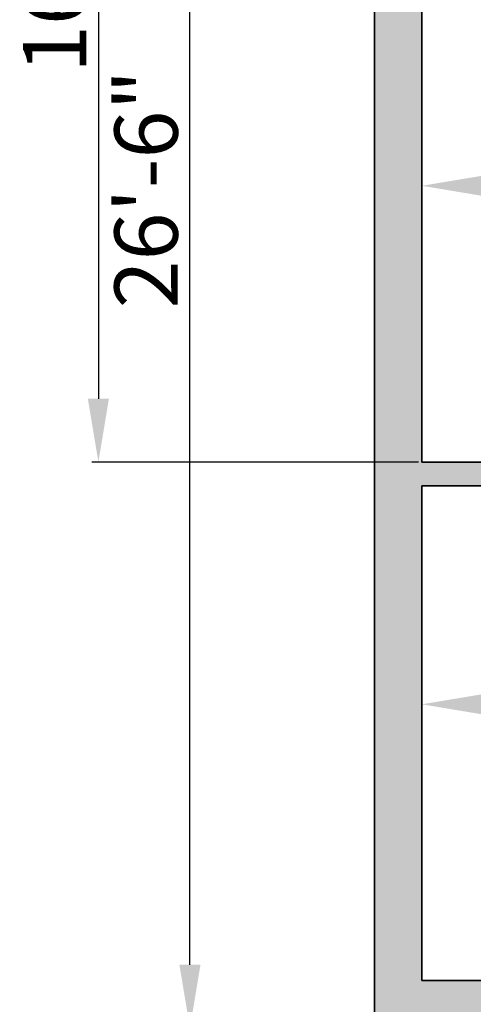
# Model space of a CAD drawing. Units: inches. Extents: x 2083 to 3317, y 1141 to 2115.
# Tile 91 of 256: x 2160 to 2246, y 1707 to 1894. Entities that reach past the tile are written whole.
import ezdxf

# ---------------------------------------------------------------- set-up
doc = ezdxf.new("R2010")
doc.units = ezdxf.units.IN
doc.layers.add('A-ANNO-DIMS', color=2, linetype='Continuous', lineweight=18)
doc.layers.add('A-WALL', color=7, linetype='Continuous', lineweight=35)
doc.layers.add('A-WALL-PATT', color=251, linetype='Continuous', lineweight=13, true_color=0x636466)
doc.styles.get("Standard").update_dxf_attribs({"font": 'arial.ttf'})
doc.dimstyles.new('ISO-25', dxfattribs={"dimtxt": 12, "dimasz": 12, "dimexe": 1.25, "dimexo": 0.625, "dimtad": 1, "dimlunit": 3, "dimtxsty": 'Standard', "dimcen": 2.5, "dimadec": 0, "dimazin": 0, "dimtfac": 1, "dimtmove": 0, "dimatfit": 3, "dimfxl": 1, "dimarcsym": 0})

# ---------------------------------------------------------------- blocks, each defined once
blk = doc.blocks.new('*D14')
at = {"layer": 'A-ANNO-DIMS', "color": 0, "lineweight": -2, "transparency": 16777216}
for p, q in [((2226.33, 2020.76), (2190.73, 2020.76)), ((2191.98, 1714.76), (2191.98, 2008.76)), ((2226.33, 1702.76), (2190.73, 1702.76))]:
    blk.add_line(p, q, dxfattribs=at)
at = {"layer": 'A-ANNO-DIMS', "color": 0, "transparency": 16777216}
for points in [[(2189.98, 2008.76), (2193.98, 2008.76), (2191.98, 2020.76)], [(2189.98, 1714.76), (2193.98, 1714.76), (2191.98, 1702.76)]]:
    blk.add_solid(points, dxfattribs=at)
at = {"layer": 'Defpoints', "color": 0, "transparency": 16777216}
for p in [(2191.98, 2020.76), (2226.96, 2020.76), (2226.96, 1702.76)]:
    blk.add_point(p, dxfattribs=at)
at = {"layer": 'A-ANNO-DIMS', "color": 0, "transparency": 16777216, "insert": (2185.22, 1861.76), "char_height": 12, "attachment_point": 5, "rotation": 90}
blk.add_mtext('26\'-6"', dxfattribs=at)
blk = doc.blocks.new('*D39')
at = {"layer": 'A-ANNO-DIMS', "color": 0, "lineweight": -2, "transparency": 16777216}
for p, q in [((2235.33, 2011.76), (2173.36, 2011.76)), ((2174.61, 1999.76), (2174.61, 1822.01)), ((2235.33, 1810.01), (2173.36, 1810.01))]:
    blk.add_line(p, q, dxfattribs=at)
at = {"layer": 'A-ANNO-DIMS', "color": 0, "transparency": 16777216}
for points in [[(2172.61, 1999.76), (2176.61, 1999.76), (2174.61, 2011.76)], [(2172.61, 1822.01), (2176.61, 1822.01), (2174.61, 1810.01)]]:
    blk.add_solid(points, dxfattribs=at)
at = {"layer": 'Defpoints', "color": 0, "transparency": 16777216}
for p in [(2235.96, 2011.76), (2174.61, 1810.01), (2235.96, 1810.01)]:
    blk.add_point(p, dxfattribs=at)
at = {"layer": 'A-ANNO-DIMS', "color": 0, "transparency": 16777216, "insert": (2167.86, 1910.89), "char_height": 12, "attachment_point": 5, "rotation": 90}
blk.add_mtext('16\'-10"', dxfattribs=at)
blk = doc.blocks.new('*D40')
at = {"layer": 'A-ANNO-DIMS', "color": 0, "lineweight": -2, "transparency": 16777216}
for p, q in [((2235.96, 1712.39), (2235.96, 1765.36)), ((2353.71, 1712.39), (2353.71, 1765.36)), ((2247.96, 1764.11), (2341.71, 1764.11))]:
    blk.add_line(p, q, dxfattribs=at)
at = {"layer": 'A-ANNO-DIMS', "color": 0, "transparency": 16777216}
for points in [[(2247.96, 1766.11), (2247.96, 1762.11), (2235.96, 1764.11)], [(2341.71, 1766.11), (2341.71, 1762.11), (2353.71, 1764.11)]]:
    blk.add_solid(points, dxfattribs=at)
at = {"layer": 'Defpoints', "color": 0, "transparency": 16777216}
for p in [(2353.71, 1764.11), (2235.96, 1711.76), (2353.71, 1711.76)]:
    blk.add_point(p, dxfattribs=at)
at = {"layer": 'A-ANNO-DIMS', "color": 0, "transparency": 16777216, "insert": (2294.83, 1770.86), "char_height": 12, "attachment_point": 5}
blk.add_mtext('9\'-10"', dxfattribs=at)
blk = doc.blocks.new('*D53')
at = {"layer": 'A-ANNO-DIMS', "color": 0, "lineweight": -2, "transparency": 16777216}
for p, q in [((2235.96, 1810.64), (2235.96, 1863.61)), ((2247.96, 1862.36), (2402.72, 1862.36)), ((2414.72, 1810.64), (2414.72, 1863.61))]:
    blk.add_line(p, q, dxfattribs=at)
at = {"layer": 'A-ANNO-DIMS', "color": 0, "transparency": 16777216}
for points in [[(2247.96, 1864.36), (2247.96, 1860.36), (2235.96, 1862.36)], [(2402.72, 1864.36), (2402.72, 1860.36), (2414.72, 1862.36)]]:
    blk.add_solid(points, dxfattribs=at)
at = {"layer": 'Defpoints', "color": 0, "transparency": 16777216}
for p in [(2414.72, 1862.36), (2235.96, 1810.01), (2414.72, 1810.01)]:
    blk.add_point(p, dxfattribs=at)
at = {"layer": 'A-ANNO-DIMS', "color": 0, "transparency": 16777216, "insert": (2325.34, 1869.01), "char_height": 12, "attachment_point": 5}
blk.add_mtext('14\'-11"', dxfattribs=at)

msp = doc.modelspace()

# ---------------------------------------------------------------- hatches: boundary and pattern name
at = {"layer": 'A-WALL-PATT'}
h = msp.add_hatch(color=256, dxfattribs=at)
h.dxf.hatch_style = 1
h.paths.add_polyline_path([(3126.96, 2020.761), (2748.96, 2020.761), (2604.96, 2020.761), (2226.96, 2020.761), (2226.96, 1702.761), (2466.96, 1702.761), (2466.96, 1582.761), (2418.96, 1582.761), (2418.96, 1477.761), (2226.96, 1477.761), (2226.96, 1263.261), (2544.96, 1263.261), (2544.96, 1411.761), (2604.96, 1411.761), (2685.96, 1411.761), (2685.96, 1420.761), (2604.96, 1420.761), (2604.96, 1573.761), (2604.96, 1702.761), (2604.96, 2011.761), (2748.96, 2011.761), (2748.96, 1702.761), (2862.96, 1702.761), (2862.96, 1621.761), (2871.96, 1621.761), (2871.96, 1702.761), (2883.96, 1702.761), (2883.96, 1706.939, -0.0264593), (2883.96, 1711.761), (2757.96, 1711.761), (2757.96, 1807.761), (2787.96, 1807.761), (2787.96, 1812.261), (2757.96, 1812.261), (2757.96, 2011.761), (2877.96, 2011.761), (2877.96, 1812.261), (2847.96, 1812.261), (2847.96, 1807.761), (2889.836, 1807.761), (2889.836, 1812.261), (2882.46, 1812.261), (2882.46, 2011.761), (3117.96, 2011.761), (3117.96, 1812.261), (2937.836, 1812.261), (2937.836, 1807.761), (2995.71, 1807.761), (2995.71, 1796.118), (3000.21, 1796.118), (3000.21, 1807.761), (3117.96, 1807.761), (3117.96, 1711.761), (3000.21, 1711.761), (3000.21, 1760.118), (2998.573, 1760.118, -0.020711), (2995.71, 1760.118), (2995.71, 1711.761), (2931.96, 1711.761), (2931.96, 1702.761), (3126.96, 1702.761)])
h.paths.add_polyline_path([(2471.46, 2011.761), (2471.46, 1810.011), (2462.717, 1810.011), (2462.717, 1805.511), (2505.96, 1805.511), (2505.96, 1810.011), (2475.96, 1810.011), (2475.96, 2011.761), (2595.96, 2011.761), (2595.96, 1810.011), (2565.96, 1810.011), (2565.96, 1805.511), (2595.96, 1805.511), (2595.96, 1711.761), (2235.96, 1711.761), (2235.96, 1805.511), (2353.71, 1805.511), (2353.71, 1796.054), (2358.21, 1796.054), (2358.21, 1805.511), (2414.717, 1805.511), (2414.717, 1810.011), (2235.96, 1810.011), (2235.96, 2011.761)], flags=16)
h.paths.add_polyline_path([(2270.205, 1994.61), (2270.205, 1970.61), (2246.205, 1970.61), (2246.205, 1994.61)], flags=0)
edge = h.paths.add_edge_path(flags=0)
edge.add_ellipse((2332.027, 1899.798), major_axis=(-3.043, 3.043), ratio=0.1682525, start_angle=-161.33217, end_angle=-156.30711, ccw=False)
edge.add_ellipse((2333.082, 1898.744), major_axis=(-1.055, 1.055), ratio=0.4535321, start_angle=-123.37102, end_angle=-94.15911)
edge = h.paths.add_edge_path(flags=0)
edge.add_ellipse((2332.027, 1968.876), major_axis=(3.043, 3.043), ratio=0.1682525, start_angle=18.66783, end_angle=23.69289)
edge.add_spline(control_points=[(2332.926, 1970.691), (2332.227, 1970.336), (2330.894, 1969.659), (2328.413, 1970.932), (2327.204, 1967.749), (2324.71, 1969.956), (2322.533, 1967.012), (2320.013, 1971.296), (2317.68, 1968.158), (2316.041, 1967.102), (2315.427, 1966.81)], knot_values=[0, 0, 0, 0, 2.2670587, 4.3245589, 6.6855835, 8.8786411, 11.121502, 14.300359, 17.7552837, 19.732645, 19.732645, 19.732645, 19.732645], degree=3, periodic=0)
edge.add_ellipse((2332.027, 1968.876), major_axis=(3.043, 3.043), ratio=0.1682525, start_angle=18.66783, end_angle=23.69289, ccw=False)
edge.add_ellipse((2333.082, 1969.931), major_axis=(1.055, 1.055), ratio=0.4535321, start_angle=56.62898, end_angle=85.84089, ccw=False)
edge = h.paths.add_edge_path(flags=0)
edge.add_spline(control_points=[(2296.428, 1967.988), (2293.628, 1965.336), (2287.704, 1959.727), (2299.744, 1949.996), (2294.533, 1935.669), (2290.573, 1920.604), (2293.394, 1909.974), (2296.185, 1904.967)], knot_values=[0.0991853, 0.0991853, 0.0991853, 0.0991853, 0.3453009, 0.6198217, 0.9826526, 1.3860932, 1.8105546, 1.8105546, 1.8105546, 1.8105546], degree=3, periodic=0)
edge.add_spline(control_points=[(2296.185, 1904.967), (2297.384, 1902.619), (2298.001, 1901.949), (2298.553, 1901.468)], knot_values=[0.0062457, 0.0062457, 0.0062457, 0.0062457, 0.0554759, 0.0554759, 0.0554759, 0.0554759], degree=3, periodic=0)
edge.add_spline(control_points=[(2298.553, 1901.468), (2297.259, 1900.923), (2295.225, 1900.232), (2293.06, 1900.614), (2292.101, 1900.788), (2292.09, 1900.791)], knot_values=[0.3128349, 0.3128349, 0.3128349, 0.3128349, 0.4017797, 0.4749867, 0.4759027, 0.4759027, 0.4759027, 0.4759027], degree=3, periodic=0)
edge.add_arc((2292.794, 1904.664), 3.937, 215.4209, 259.69818, ccw=False)
edge.add_spline(control_points=[(2289.585, 1902.382), (2289.477, 1902.535), (2289.368, 1902.688), (2289.261, 1902.841)], knot_values=[0.1028719, 0.1028719, 0.1028719, 0.1028719, 0.1168958, 0.1168958, 0.1168958, 0.1168958], degree=3, periodic=0)
edge.add_spline(control_points=[(2289.261, 1902.841), (2288.687, 1902.55), (2287.64, 1902.02), (2285.881, 1901.874), (2283.853, 1901.504), (2281.72, 1899.711), (2278.467, 1899.493), (2276.157, 1901.883), (2272.259, 1899.804), (2267.778, 1901.843), (2262.244, 1900.184), (2257.415, 1901.782), (2254.318, 1900.726), (2253.178, 1900.337)], knot_values=[0, 0, 0, 0, 1.9079767, 3.4771759, 5.261074, 7.9728515, 11.6802485, 13.7179214, 16.9395917, 22.789562, 27.5025027, 33.5952153, 37.1456181, 37.1456181, 37.1456181, 37.1456181], degree=3, periodic=0)
edge.add_line((2253.178, 1900.337), (2250.244, 1902.841))
edge.add_line((2250.244, 1902.841), (2250.244, 1965.833))
edge.add_line((2250.244, 1965.833), (2253.178, 1968.337))
edge.add_spline(control_points=[(2253.178, 1968.337), (2254.318, 1967.948), (2257.415, 1966.892), (2262.244, 1968.49), (2267.778, 1966.831), (2271.527, 1968.537), (2273.876, 1967.828), (2274.207, 1967.728)], knot_values=[0, 0, 0, 0, 0.0901802, 0.2449351, 0.3646438, 0.5132331, 0.5378548, 0.5378548, 0.5378548, 0.5378548], degree=3, periodic=0)
edge.add_arc((2274.353, 1963.793), 3.937, 72.05113, 92.12795, ccw=False)
edge.add_arc((2281.297, 1985.23), 18.596, 252.05113, 288.56572)
edge.add_arc((2292.317, 1956.029), 12.646, 71.02679, 113.77822, ccw=False)
edge = h.paths.add_edge_path(flags=0)
edge.add_spline(control_points=[(2274.899, 1951.856), (2275.066, 1951.617), (2275.233, 1951.377), (2275.398, 1951.136)], knot_values=[1.4099157, 1.4099157, 1.4099157, 1.4099157, 1.4315903, 1.4315903, 1.4315903, 1.4315903], degree=3, periodic=0)
edge.add_spline(control_points=[(2275.398, 1951.136), (2275.792, 1950.562), (2276.179, 1949.984), (2276.546, 1949.397)], knot_values=[1.3582378, 1.3582378, 1.3582378, 1.3582378, 1.4099157, 1.4099157, 1.4099157, 1.4099157], degree=3, periodic=0)
edge.add_line((2276.546, 1949.397), (2277.437, 1947.862))
edge.add_spline(control_points=[(2277.437, 1947.862), (2276.304, 1945.673), (2274.64, 1942.427), (2274.632, 1938.094), (2272.799, 1930.852), (2274.356, 1943.897), (2275.948, 1947.923), (2276.546, 1949.397)], knot_values=[0.0056315, 0.0056315, 0.0056315, 0.0056315, 0.1860139, 0.2660015, 0.3570872, 0.5963902, 0.7397317, 0.7397317, 0.7397317, 0.7397317], degree=3, periodic=0)
edge.add_spline(control_points=[(2276.546, 1949.397), (2276.179, 1949.984), (2275.792, 1950.562), (2275.398, 1951.136)], knot_values=[1.3582378, 1.3582378, 1.3582378, 1.3582378, 1.4099157, 1.4099157, 1.4099157, 1.4099157], degree=3, periodic=0)
edge.add_spline(control_points=[(2275.398, 1951.136), (2274.943, 1950.08), (2274.208, 1948.025), (2273.935, 1944.851), (2272.469, 1937.627), (2273.466, 1945.696), (2274.701, 1951.059), (2274.899, 1951.856)], knot_values=[0.1043639, 0.1043639, 0.1043639, 0.1043639, 0.1896363, 0.2696239, 0.3607096, 0.6000126, 0.6446217, 0.6446217, 0.6446217, 0.6446217], degree=3, periodic=0)
h.paths.add_polyline_path([(2269.168, 1963.128, -0.3575267), (2268.171, 1960.976, -0.0925607), (2268.171, 1939.436, -0.3575267), (2269.168, 1937.285, -0.3575267), (2267.016, 1938.282, -0.1647847), (2254.686, 1938.282, -0.3575267), (2252.534, 1937.285, -0.3575267), (2253.531, 1939.436, -0.0925607), (2253.531, 1960.976, -0.3575267), (2252.534, 1963.128, -0.3575267), (2254.686, 1962.131, -0.1647847), (2267.016, 1962.131, -0.3575267)], flags=0)
h.paths.add_polyline_path([(2248.874, 1967.802), (2248.874, 1957.028), (2249.458, 1957.028), (2249.458, 1911.647), (2248.874, 1911.647), (2248.874, 1900.873), (2246.512, 1900.873, 0.1973271), (2244.15, 1902.457), (2244.15, 1966.218, 0.1973271), (2246.512, 1967.802)], flags=0)
h.paths.add_polyline_path([(2269.168, 1931.389, -0.3575267), (2268.171, 1929.238, -0.0925607), (2268.171, 1907.698, -0.3575267), (2269.168, 1905.547, -0.3575267), (2267.016, 1906.544, -0.1647847), (2254.686, 1906.544, -0.3575267), (2252.534, 1905.547, -0.3575267), (2253.531, 1907.698, -0.0925607), (2253.531, 1929.238, -0.3575267), (2252.534, 1931.389, -0.3575267), (2254.686, 1930.392, -0.1647847), (2267.016, 1930.392, -0.3575267)], flags=0)
edge = h.paths.add_edge_path(flags=0)
edge.add_spline(control_points=[(2276.197, 1906.724), (2276.168, 1909.029), (2276.114, 1913.372), (2270.598, 1924.925), (2273.905, 1919.013), (2275.922, 1916.262), (2275.475, 1912.402), (2277.258, 1910.381), (2276.696, 1908.225), (2276.646, 1906.813), (2276.618, 1906.008)], knot_values=[0, 0, 0, 0, 8.6102597, 16.2212739, 18.8430575, 23.8048978, 27.4408283, 29.3561016, 31.2034776, 33.6506866, 33.6506866, 33.6506866, 33.6506866], degree=3, periodic=0)
edge.add_spline(control_points=[(2276.618, 1906.008), (2276.623, 1905.624), (2276.498, 1904.629), (2275.442, 1903.855), (2274.937, 1903.08), (2274.859, 1902.841)], knot_values=[0.1564884, 0.1564884, 0.1564884, 0.1564884, 0.1843975, 0.2313765, 0.2505985, 0.2505985, 0.2505985, 0.2505985], degree=3, periodic=0)
edge.add_line((2274.859, 1902.841), (2276.506, 1902.841))
edge.add_spline(control_points=[(2276.506, 1902.841), (2276.788, 1903.085), (2277.665, 1904.125), (2278.25, 1904.341), (2277.654, 1908.527), (2278.156, 1906.228), (2278.1, 1905.286), (2278.847, 1904.069), (2277.857, 1903.415), (2277.874, 1902.991), (2277.904, 1902.841)], knot_values=[0.0595743, 0.0595743, 0.0595743, 0.0595743, 0.0807529, 0.1037415, 0.1697201, 0.1760361, 0.2071372, 0.2404744, 0.2623409, 0.2736605, 0.2736605, 0.2736605, 0.2736605], degree=3, periodic=0)
edge.add_line((2277.904, 1902.841), (2280.03, 1902.841))
edge.add_spline(control_points=[(2280.03, 1902.841), (2279.888, 1903.088), (2279.499, 1903.982), (2280.152, 1905.939), (2278.104, 1909.658), (2279.762, 1907.185), (2280.328, 1904.875), (2280.485, 1903.49), (2281.463, 1903.249), (2281.758, 1902.936), (2281.834, 1902.841)], knot_values=[0.013856, 0.013856, 0.013856, 0.013856, 0.0348738, 0.0888667, 0.1078792, 0.1267378, 0.158714, 0.1937575, 0.2174868, 0.2267221, 0.2267221, 0.2267221, 0.2267221], degree=3, periodic=0)
edge.add_spline(control_points=[(2281.834, 1902.841), (2281.788, 1902.827), (2281.647, 1902.783), (2281.396, 1902.859), (2281.088, 1902.985), (2280.721, 1903.061), (2280.333, 1903.026), (2280.125, 1902.899), (2280.03, 1902.841)], knot_values=[0, 0, 0, 0, 0.1441304, 0.435517, 0.7492759, 1.1530457, 1.5483707, 1.878348, 1.878348, 1.878348, 1.878348], degree=3, periodic=0)
edge.add_line((2280.03, 1902.841), (2277.904, 1902.841))
edge.add_spline(control_points=[(2277.904, 1902.841), (2277.893, 1902.796), (2277.865, 1902.68), (2277.607, 1902.687), (2277.274, 1902.801), (2276.838, 1902.62), (2276.584, 1902.789), (2276.506, 1902.841)], knot_values=[0, 0, 0, 0, 0.1271885, 0.3261988, 0.6280094, 1.2435704, 1.5153306, 1.5153306, 1.5153306, 1.5153306], degree=3, periodic=0)
edge.add_line((2276.506, 1902.841), (2274.859, 1902.841))
edge.add_spline(control_points=[(2274.859, 1902.841), (2274.814, 1902.899), (2274.725, 1903.013), (2274.493, 1903.119), (2274.244, 1902.961), (2273.937, 1903.185), (2273.614, 1902.983), (2273.408, 1902.883), (2273.322, 1902.841)], knot_values=[0, 0, 0, 0, 0.2184302, 0.4369566, 0.6879766, 0.9903786, 1.3983955, 1.6918498, 1.6918498, 1.6918498, 1.6918498], degree=3, periodic=0)
edge.add_spline(control_points=[(2273.322, 1902.841), (2273.617, 1903.446), (2274.274, 1904.538), (2276.027, 1904.574), (2276.207, 1906.584), (2276.197, 1906.724)], knot_values=[0.0122268, 0.0122268, 0.0122268, 0.0122268, 0.0594721, 0.1062177, 0.134458, 0.134458, 0.134458, 0.134458], degree=3, periodic=0)
h.paths.add_polyline_path([(2270.776, 1897.79), (2270.776, 1873.79), (2246.776, 1873.79), (2246.776, 1897.79)], flags=0)
h.paths.add_polyline_path([(2353.71, 1760.005), (2353.71, 1760.054), (2358.21, 1760.054, -0.033729)], flags=0)
h.paths.add_polyline_path([(2321.819, 1737.529), (2341.995, 1737.529, -0.4142136), (2343.203, 1736.321), (2343.203, 1721.021, -0.4142136), (2341.995, 1719.813), (2321.819, 1719.813, -0.4142136), (2320.611, 1721.021), (2320.611, 1736.321, -0.4142136)], flags=0)
h.paths.add_polyline_path([(2324.235, 1736.321), (2339.579, 1736.321, -0.4142136), (2341.995, 1733.905), (2341.995, 1725.45, -0.4142136), (2339.579, 1723.034), (2333.681, 1723.034), (2333.845, 1722.045, -0.8706461), (2335.425, 1721.826, -0.767327), (2333.923, 1721.423), (2331.291, 1721.423, -0.767327), (2329.788, 1721.826, -0.8706461), (2331.368, 1722.045), (2331.533, 1723.034), (2324.235, 1723.034, -0.4142136), (2321.819, 1725.45), (2321.819, 1733.905, -0.4142136)], flags=0)
h.paths.add_polyline_path([(2570.484, 1928.615), (2589.684, 1928.615), (2590.169, 1928.615), (2590.169, 1904.993), (2570.484, 1904.993)], flags=0)
h.paths.add_polyline_path([(2574.447, 1927.264, -1), (2572.829, 1927.264, -1)], flags=0)
h.paths.add_polyline_path([(2573.09, 1926.941), (2573.925, 1927.776), (2574.148, 1927.553), (2573.313, 1926.718)], flags=0)
h.paths.add_polyline_path([(2578.779, 1919.73, -1), (2571.592, 1919.73, -1)], flags=0)
h.paths.add_polyline_path([(2578.385, 1919.73, -1), (2571.985, 1919.73, -1)], flags=0)
h.paths.add_polyline_path([(2331.596, 1729.476, -1), (2333.618, 1729.476, -1)], flags=0)
h.paths.add_polyline_path([(2578.034, 1927.264, -1), (2576.416, 1927.264, -1)], flags=0)
h.paths.add_polyline_path([(2576.689, 1927.531), (2576.912, 1927.754), (2577.747, 1926.919), (2577.524, 1926.696)], flags=0)
h.paths.add_polyline_path([(2578.139, 1909.86, -1), (2572.232, 1909.86, -1)], flags=0)
h.paths.add_polyline_path([(2577.745, 1909.86, -1), (2572.625, 1909.86, -1)], flags=0)
h.paths.add_polyline_path([(2583.798, 1927.264, -1), (2582.179, 1927.264, -1)], flags=0)
h.paths.add_polyline_path([(2582.719, 1927.754), (2583.554, 1926.919), (2583.331, 1926.696), (2582.496, 1927.531)], flags=0)
h.paths.add_polyline_path([(2582.496, 1927.531), (2582.719, 1927.754), (2583.554, 1926.919), (2583.331, 1926.696)], flags=0)
h.paths.add_polyline_path([(2587.739, 1920.53, -1), (2581.832, 1920.53, -1)], flags=0)
h.paths.add_polyline_path([(2587.345, 1920.53, -1), (2582.225, 1920.53, -1)], flags=0)
h.paths.add_polyline_path([(2587.385, 1927.264, -1), (2585.766, 1927.264, -1)], flags=0)
h.paths.add_polyline_path([(2586.082, 1926.98), (2586.917, 1927.815), (2587.14, 1927.593), (2586.305, 1926.758)], flags=0)
h.paths.add_polyline_path([(2588.379, 1910.66, -1), (2581.192, 1910.66, -1)], flags=0)
h.paths.add_polyline_path([(2587.985, 1910.66, -1), (2581.585, 1910.66, -1)], flags=0)
h.paths.add_polyline_path([(2417.168, 1729.478), (2437.344, 1729.478, -0.4142136), (2438.552, 1728.27), (2438.552, 1712.969, -0.4142136), (2437.344, 1711.761), (2417.168, 1711.761, -0.4142136), (2415.96, 1712.969), (2415.96, 1728.27, -0.4142136)], flags=0)
h.paths.add_polyline_path([(2419.584, 1728.27), (2434.928, 1728.27, -0.4142136), (2437.344, 1725.854), (2437.344, 1717.398, -0.4142136), (2434.928, 1714.983), (2429.029, 1714.983), (2429.194, 1713.994, -0.8706461), (2430.774, 1713.775, -0.767327), (2429.271, 1713.372), (2426.64, 1713.372, -0.767327), (2425.137, 1713.775, -0.8706461), (2426.717, 1713.994), (2426.882, 1714.983), (2419.584, 1714.983, -0.4142136), (2417.168, 1717.398), (2417.168, 1725.854, -0.4142136)], flags=0)
h.paths.add_polyline_path([(2419.584, 1728.27), (2434.928, 1728.27, -0.4142136), (2437.344, 1725.854), (2437.344, 1717.398, -0.4142136), (2434.928, 1714.983), (2429.029, 1714.983), (2428.358, 1719.009), (2427.553, 1719.009), (2426.882, 1714.983), (2419.584, 1714.983, -0.4142136), (2417.168, 1717.398), (2417.168, 1725.854, -0.4142136)], flags=0)
h.paths.add_polyline_path([(2426.944, 1721.425, -1), (2428.967, 1721.425, -1)], flags=0)
h.paths.add_polyline_path([(2475.96, 1702.761), (2595.96, 1702.761), (2595.96, 1582.761), (2475.96, 1582.761)], flags=16)
h.paths.add_polyline_path([(2427.96, 1573.761), (2595.96, 1573.761), (2595.96, 1468.761), (2595.96, 1420.761), (2384.46, 1420.761), (2384.46, 1468.761), (2427.96, 1468.761)], flags=16)
h.paths.add_polyline_path([(2379.96, 1468.761), (2379.96, 1420.761), (2235.96, 1420.761), (2235.96, 1468.761)], flags=16)
h.paths.add_polyline_path([(2317.816, 1466.696), (2337.992, 1466.696, -0.4142136), (2339.2, 1465.488), (2339.2, 1450.187, -0.4142136), (2337.992, 1448.979), (2317.816, 1448.979, -0.4142136), (2316.608, 1450.187), (2316.608, 1465.488, -0.4142136)], flags=0)
h.paths.add_polyline_path([(2320.232, 1465.488), (2335.576, 1465.488, -0.4142136), (2337.992, 1463.072), (2337.992, 1454.616, -0.4142136), (2335.576, 1452.2), (2329.677, 1452.2), (2329.842, 1451.212, -0.8706461), (2331.422, 1450.992, -0.767327), (2329.92, 1450.59), (2327.288, 1450.59, -0.767327), (2325.785, 1450.992, -0.8706461), (2327.365, 1451.212), (2327.53, 1452.2), (2320.232, 1452.2, -0.4142136), (2317.816, 1454.616), (2317.816, 1463.072, -0.4142136)], flags=0)
h.paths.add_polyline_path([(2320.232, 1465.488), (2335.576, 1465.488, -0.4142136), (2337.992, 1463.072), (2337.992, 1454.616, -0.4142136), (2335.576, 1452.2), (2329.677, 1452.2), (2329.006, 1456.227), (2328.201, 1456.227), (2327.53, 1452.2), (2320.232, 1452.2, -0.4142136), (2317.816, 1454.616), (2317.816, 1463.072, -0.4142136)], flags=0)
h.paths.add_polyline_path([(2327.593, 1458.643, -1), (2329.615, 1458.643, -1)], flags=0)
h.paths.add_polyline_path([(2244.412, 1433.34), (2241.921, 1433.34, -0.4142136), (2240.018, 1435.244), (2240.018, 1440.953, -0.4142105), (2241.921, 1442.856), (2244.412, 1442.856, -1.9764724)], flags=0)
h.paths.add_polyline_path([(2245.357, 1434.398, -0.4142136), (2245.357, 1441.799, -2.1440985)], flags=0)
h.paths.add_polyline_path([(2535.96, 1416.261), (2535.96, 1272.261), (2235.96, 1272.261), (2235.96, 1416.261)], flags=16)
h.paths.add_polyline_path([(2260.12, 1384.293), (2260.12, 1362.039), (2237.865, 1362.039), (2237.865, 1384.293)], flags=0)
edge = h.paths.add_edge_path(flags=0)
edge.add_line((2318.252, 1362.093), (2318.146, 1362.001))
edge.add_ellipse((2317.445, 1360.431), major_axis=(2.822, 2.822), ratio=0.1682525, start_angle=18.66783, end_angle=20.94813, ccw=False)
edge.add_ellipse((2318.423, 1361.409), major_axis=(0.978, 0.978), ratio=0.4535321, start_angle=56.62898, end_angle=70.2262, ccw=False)
edge = h.paths.add_edge_path(flags=0)
edge.add_line((2319.107, 1295.571), (2319.015, 1295.677))
edge.add_ellipse((2317.445, 1296.378), major_axis=(-2.822, 2.822), ratio=0.1682525, start_angle=-161.33217, end_angle=-159.05187, ccw=False)
edge.add_ellipse((2318.423, 1295.4), major_axis=(-0.978, 0.978), ratio=0.4535321, start_angle=-123.37102, end_angle=-109.7738)
edge = h.paths.add_edge_path(flags=0)
edge.add_spline(control_points=[(2284.21, 1301.17), (2284.581, 1300.445), (2284.891, 1299.892), (2285.16, 1299.461)], knot_values=[0.0390658, 0.0390658, 0.0390658, 0.0390658, 0.0554759, 0.0554759, 0.0554759, 0.0554759], degree=3, periodic=0)
edge.add_line((2285.16, 1299.461), (2284.21, 1301.17))
edge = h.paths.add_edge_path(flags=0)
edge.add_line((2280.412, 1297.298), (2283.37, 1297.036))
edge.add_line((2283.37, 1297.036), (2286.406, 1297.926))
edge.add_spline(control_points=[(2286.406, 1297.926), (2285.305, 1297.463), (2284.345, 1297.129), (2283.37, 1297.036)], knot_values=[0.3943688, 0.3943688, 0.3943688, 0.3943688, 0.4759027, 0.4759027, 0.4759027, 0.4759027], degree=3, periodic=0)
edge.add_spline(control_points=[(2283.37, 1297.036), (2283.281, 1297.028), (2282.316, 1296.957), (2281.313, 1297.134), (2280.423, 1297.296), (2280.412, 1297.298)], knot_values=[0.3128349, 0.3128349, 0.3128349, 0.3128349, 0.3202458, 0.3934528, 0.3943688, 0.3943688, 0.3943688, 0.3943688], degree=3, periodic=0)
edge = h.paths.add_edge_path(flags=0)
edge.add_line((2284.436, 1359.607), (2280.446, 1355.328))
edge.add_line((2280.446, 1355.328), (2279.58, 1351.018))
edge.add_line((2279.58, 1351.018), (2282.413, 1346.58))
edge.add_spline(control_points=[(2282.413, 1346.58), (2283.153, 1345.589), (2284.253, 1344.029), (2284.801, 1342.387), (2284.935, 1341.806)], knot_values=[1.2400982, 1.2400982, 1.2400982, 1.2400982, 1.3328922, 1.3827123, 1.3827123, 1.3827123, 1.3827123], degree=3, periodic=0)
edge.add_spline(control_points=[(2284.935, 1341.806), (2285.319, 1340.141), (2285.233, 1338.409), (2284.91, 1336.654)], knot_values=[1.0974841, 1.0974841, 1.0974841, 1.0974841, 1.2400982, 1.2400982, 1.2400982, 1.2400982], degree=3, periodic=0)
edge.add_spline(control_points=[(2284.91, 1336.654), (2284.587, 1334.899), (2284.027, 1333.12), (2283.463, 1331.361)], knot_values=[0.9548699, 0.9548699, 0.9548699, 0.9548699, 1.0974841, 1.0974841, 1.0974841, 1.0974841], degree=3, periodic=0)
edge.add_line((2283.463, 1331.361), (2281.89, 1326.153))
edge.add_line((2281.89, 1326.153), (2280.756, 1321.056))
edge.add_line((2280.756, 1321.056), (2280.299, 1316.002))
edge.add_line((2280.299, 1316.002), (2280.716, 1310.95))
edge.add_line((2280.716, 1310.95), (2282.028, 1305.972))
edge.add_line((2282.028, 1305.972), (2284.21, 1301.17))
edge.add_spline(control_points=[(2284.21, 1301.17), (2283.341, 1302.73), (2282.612, 1304.336), (2282.028, 1305.972)], knot_values=[0.0991853, 0.0991853, 0.0991853, 0.0991853, 0.2417994, 0.2417994, 0.2417994, 0.2417994], degree=3, periodic=0)
edge.add_spline(control_points=[(2282.028, 1305.972), (2281.444, 1307.608), (2281.005, 1309.273), (2280.716, 1310.95)], knot_values=[0.2417994, 0.2417994, 0.2417994, 0.2417994, 0.3844135, 0.3844135, 0.3844135, 0.3844135], degree=3, periodic=0)
edge.add_spline(control_points=[(2280.716, 1310.95), (2280.433, 1312.588), (2280.289, 1314.277), (2280.299, 1315.962), (2280.299, 1316.002)], knot_values=[0.3844135, 0.3844135, 0.3844135, 0.3844135, 0.5236467, 0.5270276, 0.5270276, 0.5270276, 0.5270276], degree=3, periodic=0)
edge.add_spline(control_points=[(2280.299, 1316.002), (2280.312, 1317.687), (2280.478, 1319.368), (2280.756, 1321.056)], knot_values=[0.5270276, 0.5270276, 0.5270276, 0.5270276, 0.6696417, 0.6696417, 0.6696417, 0.6696417], degree=3, periodic=0)
edge.add_spline(control_points=[(2280.756, 1321.056), (2281.035, 1322.744), (2281.426, 1324.44), (2281.89, 1326.153)], knot_values=[0.6696417, 0.6696417, 0.6696417, 0.6696417, 0.8122558, 0.8122558, 0.8122558, 0.8122558], degree=3, periodic=0)
edge.add_spline(control_points=[(2281.89, 1326.153), (2282.264, 1327.533), (2282.788, 1329.262), (2283.353, 1331.018), (2283.463, 1331.361)], knot_values=[0.8122558, 0.8122558, 0.8122558, 0.8122558, 0.9270873, 0.9548699, 0.9548699, 0.9548699, 0.9548699], degree=3, periodic=0)
edge.add_line((2283.463, 1331.361), (2284.91, 1336.654))
edge.add_line((2284.91, 1336.654), (2284.935, 1341.806))
edge.add_line((2284.935, 1341.806), (2282.413, 1346.58))
edge.add_spline(control_points=[(2282.413, 1346.58), (2281.275, 1348.104), (2280.078, 1349.57), (2279.58, 1351.018)], knot_values=[1.3827123, 1.3827123, 1.3827123, 1.3827123, 1.5253264, 1.5253264, 1.5253264, 1.5253264], degree=3, periodic=0)
edge.add_spline(control_points=[(2279.58, 1351.018), (2279.443, 1351.415), (2279.136, 1352.857), (2279.735, 1354.29), (2280.446, 1355.328)], knot_values=[1.5253264, 1.5253264, 1.5253264, 1.5253264, 1.564439, 1.6679405, 1.6679405, 1.6679405, 1.6679405], degree=3, periodic=0)
edge.add_spline(control_points=[(2280.446, 1355.328), (2281.426, 1356.758), (2282.931, 1358.183), (2284.436, 1359.607)], knot_values=[1.6679405, 1.6679405, 1.6679405, 1.6679405, 1.8105546, 1.8105546, 1.8105546, 1.8105546], degree=3, periodic=0)
edge.add_arc((2280.623, 1348.518), 11.726, 71.02679, 113.77822)
edge.add_arc((2270.405, 1375.595), 17.244, 252.05113, 288.56572, ccw=False)
edge.add_arc((2263.966, 1355.718), 3.651, 72.05113, 92.12795)
edge.add_arc((2263.966, 1355.718), 3.651, 92.12795, 177.98513)
edge.add_spline(control_points=[(2260.318, 1355.846), (2260.26, 1354.221), (2260.551, 1350.187), (2262.999, 1346.766), (2264.473, 1344.649)], knot_values=[1.4315903, 1.4315903, 1.4315903, 1.4315903, 1.5641438, 1.7706953, 1.7706953, 1.7706953, 1.7706953], degree=3, periodic=0)
edge.add_line((2264.473, 1344.649), (2264.936, 1343.983))
edge.add_spline(control_points=[(2263.801, 1340.248), (2263.843, 1340.514), (2264.067, 1341.756), (2264.513, 1343.002), (2264.935, 1343.981)], knot_values=[0.5365702, 0.5365702, 0.5365702, 0.5365702, 0.5593494, 0.6446217, 0.6446217, 0.6446217, 0.6446217], degree=3, periodic=0)
edge.add_spline(control_points=[(2264.935, 1343.981), (2265.118, 1343.715), (2265.299, 1343.448), (2265.477, 1343.179)], knot_values=[1.3840767, 1.3840767, 1.3840767, 1.3840767, 1.4099157, 1.4099157, 1.4099157, 1.4099157], degree=3, periodic=0)
edge.add_spline(control_points=[(2265.477, 1343.179), (2265.655, 1342.911), (2265.829, 1342.641), (2265.999, 1342.369)], knot_values=[1.3582378, 1.3582378, 1.3582378, 1.3582378, 1.3840767, 1.3840767, 1.3840767, 1.3840767], degree=3, periodic=0)
edge.add_line((2265.999, 1342.369), (2266.826, 1340.946))
edge.add_spline(control_points=[(2266.826, 1340.946), (2268.894, 1337.09), (2271.398, 1325.843), (2270.516, 1310.569), (2275.919, 1301.861), (2277.79, 1299.199)], knot_values=[0.1168958, 0.1168958, 0.1168958, 0.1168958, 0.4729873, 1.0509689, 1.3137934, 1.3137934, 1.3137934, 1.3137934], degree=3, periodic=0)
edge.add_spline(control_points=[(2277.79, 1299.199), (2277.839, 1299.128), (2277.889, 1299.057), (2277.94, 1298.987)], knot_values=[0.1098839, 0.1098839, 0.1098839, 0.1098839, 0.1168958, 0.1168958, 0.1168958, 0.1168958], degree=3, periodic=0)
edge.add_line((2277.94, 1298.987), (2277.789, 1299.199))
edge.add_spline(control_points=[(2277.789, 1299.199), (2277.257, 1298.929), (2276.286, 1298.438), (2275.039, 1298.334), (2274.383, 1298.239), (2274.215, 1298.209)], knot_values=[33.1218702, 33.1218702, 33.1218702, 33.1218702, 35.0290557, 36.5982549, 37.1448269, 37.1448269, 37.1448269, 37.1448269], degree=3, periodic=0)
edge.add_line((2274.215, 1298.209), (2273.073, 1297.893))
edge.add_spline(control_points=[(2273.073, 1297.893), (2272.323, 1297.58), (2271.039, 1296.511), (2269.248, 1296.226), (2268.423, 1296.375)], knot_values=[26.5325843, 26.5325843, 26.5325843, 26.5325843, 29.198919, 31.8391012, 31.8391012, 31.8391012, 31.8391012], degree=3, periodic=0)
edge.add_line((2268.423, 1296.375), (2263.879, 1297.458))
edge.add_spline(control_points=[(2263.879, 1297.458), (2263.556, 1297.359), (2261.86, 1296.839), (2260.239, 1297.282), (2258.933, 1297.516)], knot_values=[15.9195506, 15.9195506, 15.9195506, 15.9195506, 16.9395917, 21.2260675, 21.2260675, 21.2260675, 21.2260675], degree=3, periodic=0)
edge.add_line((2258.933, 1297.516), (2254.055, 1297.329))
edge.add_spline(control_points=[(2254.055, 1297.329), (2253.756, 1297.296), (2252.114, 1297.165), (2250.462, 1297.544), (2249.13, 1297.668)], knot_values=[5.3065169, 5.3065169, 5.3065169, 5.3065169, 6.2764352, 10.6130337, 10.6130337, 10.6130337, 10.6130337], degree=3, periodic=0)
edge.add_line((2249.13, 1297.668), (2244.332, 1296.878))
edge.add_line((2244.332, 1296.878), (2241.611, 1299.199))
edge.add_line((2241.611, 1299.199), (2241.611, 1357.609))
edge.add_line((2241.611, 1357.609), (2244.332, 1359.931))
edge.add_line((2244.332, 1359.931), (2252.729, 1359.543))
edge.add_spline(control_points=[(2252.729, 1359.543), (2252.871, 1359.546), (2253.306, 1359.548), (2253.74, 1359.514), (2254.032, 1359.482)], knot_values=[0.233291, 0.233291, 0.233291, 0.233291, 0.2449351, 0.2689274, 0.2689274, 0.2689274, 0.2689274], degree=3, periodic=0)
edge.add_line((2254.032, 1359.482), (2259.587, 1359.416))
edge.add_spline(control_points=[(2259.587, 1359.416), (2260.677, 1359.629), (2262.073, 1359.897), (2263.524, 1359.459), (2263.83, 1359.366)], knot_values=[0.4225164, 0.4225164, 0.4225164, 0.4225164, 0.5132331, 0.5378548, 0.5378548, 0.5378548, 0.5378548], degree=3, periodic=0)
edge.add_arc((2263.966, 1355.718), 3.651, 72.05113, 92.12795, ccw=False)
edge.add_arc((2270.405, 1375.595), 17.244, 252.05113, 288.56572)
edge.add_arc((2280.623, 1348.518), 11.726, 71.02679, 113.77822, ccw=False)
h.paths.add_polyline_path([(2240.341, 1359.435), (2240.341, 1349.444), (2240.882, 1349.444), (2240.882, 1307.365), (2240.341, 1307.365), (2240.341, 1297.374), (2238.15, 1297.374, 0.1973271), (2235.96, 1298.843), (2235.96, 1357.966, 0.1973271), (2238.15, 1359.435)], flags=0)
h.paths.add_polyline_path([(2259.158, 1355.101, -0.3575267), (2258.233, 1353.106, -0.0925607), (2258.233, 1333.133, -0.3575267), (2259.158, 1331.138, -0.3575267), (2257.163, 1332.062, -0.1647847), (2245.729, 1332.062, -0.3575267), (2243.735, 1331.138, -0.3575267), (2244.659, 1333.133, -0.0925607), (2244.659, 1353.106, -0.3575267), (2243.735, 1355.101, -0.3575267), (2245.729, 1354.176, -0.1647847), (2257.163, 1354.176, -0.3575267)], flags=0)
edge = h.paths.add_edge_path(flags=0)
edge.add_line((2265.999, 1342.369), (2266.826, 1340.946))
edge.add_line((2266.826, 1340.946), (2265.308, 1337.814))
edge.add_line((2265.308, 1337.814), (2264.358, 1334.653))
edge.add_line((2264.358, 1334.653), (2264.262, 1333.8))
edge.add_spline(control_points=[(2264.262, 1333.8), (2264.208, 1333.187), (2264.162, 1332.366), (2264.007, 1331.414), (2263.969, 1331.202)], knot_values=[0.4644442, 0.4644442, 0.4644442, 0.4644442, 0.5166905, 0.5316081, 0.5316081, 0.5316081, 0.5316081], degree=3, periodic=0)
edge.add_spline(control_points=[(2263.969, 1331.202), (2263.775, 1330.119), (2263.424, 1328.791), (2263.257, 1328.531), (2263.234, 1328.515)], knot_values=[0.3726816, 0.3726816, 0.3726816, 0.3726816, 0.4488497, 0.4644442, 0.4644442, 0.4644442, 0.4644442], degree=3, periodic=0)
edge.add_spline(control_points=[(2263.234, 1328.515), (2263.096, 1328.42), (2263.131, 1329.301), (2263.275, 1330.616)], knot_values=[0.2809191, 0.2809191, 0.2809191, 0.2809191, 0.3726816, 0.3726816, 0.3726816, 0.3726816], degree=3, periodic=0)
edge.add_spline(control_points=[(2263.275, 1330.616), (2263.419, 1331.93), (2263.672, 1333.677), (2263.97, 1335.315)], knot_values=[0.1891566, 0.1891566, 0.1891566, 0.1891566, 0.2809191, 0.2809191, 0.2809191, 0.2809191], degree=3, periodic=0)
edge.add_spline(control_points=[(2263.97, 1335.315), (2264.1, 1336.032), (2264.419, 1337.622), (2264.755, 1338.864), (2264.947, 1339.491)], knot_values=[0.097394, 0.097394, 0.097394, 0.097394, 0.1375775, 0.1891566, 0.1891566, 0.1891566, 0.1891566], degree=3, periodic=0)
edge.add_spline(control_points=[(2264.947, 1339.491), (2265.29, 1340.606), (2265.644, 1341.494), (2265.999, 1342.369)], knot_values=[0.0056315, 0.0056315, 0.0056315, 0.0056315, 0.097394, 0.097394, 0.097394, 0.097394], degree=3, periodic=0)
h.paths.add_polyline_path([(2259.158, 1325.671, -0.3575267), (2258.233, 1323.676, -0.0925607), (2258.233, 1303.703, -0.3575267), (2259.158, 1301.708, -0.3575267), (2257.163, 1302.633, -0.1647847), (2245.729, 1302.633, -0.3575267), (2243.735, 1301.708, -0.3575267), (2244.659, 1303.703, -0.0925607), (2244.659, 1323.676, -0.3575267), (2243.735, 1325.671, -0.3575267), (2245.729, 1324.747, -0.1647847), (2257.163, 1324.747, -0.3575267)], flags=0)
edge = h.paths.add_edge_path(flags=0)
edge.add_spline(control_points=[(2261.709, 1317.311), (2261.679, 1317.418), (2261.762, 1317.389), (2262.491, 1316.09), (2262.962, 1315.301)], knot_values=[14.9558607, 14.9558607, 14.9558607, 14.9558607, 16.2212739, 18.6948259, 18.6948259, 18.6948259, 18.6948259], degree=3, periodic=0)
edge.add_spline(control_points=[(2262.962, 1315.301), (2262.99, 1315.254), (2263.702, 1314.067), (2264.349, 1313.127), (2264.73, 1312.164)], knot_values=[18.6948259, 18.6948259, 18.6948259, 18.6948259, 18.8430575, 22.433791, 22.433791, 22.433791, 22.433791], degree=3, periodic=0)
edge.add_spline(control_points=[(2264.73, 1312.164), (2264.876, 1311.796), (2265.177, 1310.77), (2265.143, 1309.559), (2265.248, 1308.824)], knot_values=[22.433791, 22.433791, 22.433791, 22.433791, 23.8048978, 26.1727562, 26.1727562, 26.1727562, 26.1727562], degree=3, periodic=0)
edge.add_line((2265.248, 1308.824), (2265.851, 1307.172))
edge.add_spline(control_points=[(2265.851, 1307.172), (2266.065, 1306.822), (2266.384, 1306.332), (2266.424, 1305.781), (2266.42, 1305.611)], knot_values=[28.0625624, 28.0625624, 28.0625624, 28.0625624, 29.3561016, 29.9117214, 29.9117214, 29.9117214, 29.9117214], degree=3, periodic=0)
edge.add_spline(control_points=[(2266.42, 1305.611), (2266.416, 1305.433), (2266.394, 1305.25), (2266.365, 1305.066)], knot_values=[29.9117214, 29.9117214, 29.9117214, 29.9117214, 30.4978371, 30.4978371, 30.4978371, 30.4978371], degree=3, periodic=0)
edge.add_line((2266.365, 1305.066), (2266.066, 1302.136))
edge.add_spline(control_points=[(2266.066, 1302.136), (2266.071, 1301.78), (2265.998, 1301.2), (2265.663, 1300.759), (2265.509, 1300.586)], knot_values=[0.1564884, 0.1564884, 0.1564884, 0.1564884, 0.1843975, 0.2035434, 0.2035434, 0.2035434, 0.2035434], degree=3, periodic=0)
edge.add_line((2265.509, 1300.586), (2264.435, 1299.199))
edge.add_line((2264.435, 1299.199), (2265.962, 1299.199))
edge.add_line((2265.962, 1299.199), (2267.336, 1301.175))
edge.add_line((2267.336, 1301.175), (2267.312, 1301.986))
edge.add_spline(control_points=[(2267.312, 1301.986), (2267.261, 1302.862), (2267.16, 1303.737), (2267.271, 1303.326)], knot_values=[0.1262286, 0.1262286, 0.1262286, 0.1262286, 0.1666174, 0.1666174, 0.1666174, 0.1666174], degree=3, periodic=0)
edge.add_spline(control_points=[(2267.271, 1303.326), (2267.28, 1303.294), (2267.31, 1303.175), (2267.373, 1302.884), (2267.406, 1302.683), (2267.418, 1302.601)], knot_values=[0.1666174, 0.1666174, 0.1666174, 0.1666174, 0.1697201, 0.1760361, 0.1807647, 0.1807647, 0.1807647, 0.1807647], degree=3, periodic=0)
edge.add_spline(control_points=[(2267.744, 1300.988), (2267.688, 1301.151), (2267.481, 1301.657), (2267.484, 1302.145), (2267.418, 1302.601)], knot_values=[0.1807647, 0.1807647, 0.1807647, 0.1807647, 0.1937665, 0.2201389, 0.2201389, 0.2201389, 0.2201389], degree=3, periodic=0)
edge.add_line((2267.418, 1302.601), (2267.744, 1300.988))
edge.add_spline(control_points=[(2267.744, 1300.988), (2267.832, 1300.732), (2267.932, 1300.31), (2267.555, 1299.975), (2267.429, 1299.829)], knot_values=[0.2201389, 0.2201389, 0.2201389, 0.2201389, 0.2404744, 0.2548903, 0.2548903, 0.2548903, 0.2548903], degree=3, periodic=0)
edge.add_line((2267.429, 1299.829), (2267.258, 1299.199))
edge.add_line((2267.258, 1299.199), (2269.23, 1299.199))
edge.add_spline(control_points=[(2269.23, 1299.199), (2269.099, 1299.429), (2268.843, 1300.016), (2269.012, 1300.916), (2268.947, 1301.661)], knot_values=[0.013856, 0.013856, 0.013856, 0.013856, 0.0348738, 0.0670726, 0.0670726, 0.0670726, 0.0670726], degree=3, periodic=0)
edge.add_line((2268.947, 1301.661), (2268.432, 1303.603))
edge.add_spline(control_points=[(2268.432, 1303.603), (2268.176, 1304.192), (2267.596, 1305.251), (2268.041, 1304.623), (2268.251, 1304.282)], knot_values=[0.0901547, 0.0901547, 0.0901547, 0.0901547, 0.1078792, 0.1202891, 0.1202891, 0.1202891, 0.1202891], degree=3, periodic=0)
edge.add_spline(control_points=[(2268.251, 1304.282), (2268.361, 1304.105), (2269.058, 1302.918), (2269.383, 1301.59), (2269.521, 1300.776), (2269.575, 1300.556)], knot_values=[0.1202891, 0.1202891, 0.1202891, 0.1202891, 0.1267378, 0.158714, 0.1735056, 0.1735056, 0.1735056, 0.1735056], degree=3, periodic=0)
edge.add_line((2269.575, 1300.556), (2270.686, 1299.421))
edge.add_spline(control_points=[(2270.686, 1299.421), (2270.767, 1299.357), (2270.838, 1299.281), (2270.903, 1299.199)], knot_values=[0.2181597, 0.2181597, 0.2181597, 0.2181597, 0.2267221, 0.2267221, 0.2267221, 0.2267221], degree=3, periodic=0)
edge.add_line((2270.937, 1299.193), (2270.903, 1299.199))
edge.add_spline(control_points=[(2270.903, 1299.199), (2270.86, 1299.186), (2270.73, 1299.146), (2270.496, 1299.216), (2270.272, 1299.308), (2270.121, 1299.348), (2270.063, 1299.36)], knot_values=[0.939174, 0.939174, 0.939174, 0.939174, 1.0833044, 1.3746911, 1.6884499, 1.878348, 1.878348, 1.878348, 1.878348], degree=3, periodic=0)
edge.add_line((2270.063, 1299.36), (2269.23, 1299.199))
edge.add_line((2269.23, 1299.199), (2267.258, 1299.199))
edge.add_spline(control_points=[(2267.258, 1299.199), (2267.248, 1299.157), (2267.223, 1299.05), (2266.984, 1299.057), (2266.809, 1299.116), (2266.677, 1299.109), (2266.637, 1299.105)], knot_values=[0.7576653, 0.7576653, 0.7576653, 0.7576653, 0.8848538, 1.0838641, 1.3856747, 1.5153306, 1.5153306, 1.5153306, 1.5153306], degree=3, periodic=0)
edge.add_spline(control_points=[(2266.637, 1299.105), (2266.485, 1299.089), (2266.236, 1299.017), (2266.035, 1299.151), (2265.962, 1299.199)], knot_values=[0, 0, 0, 0, 0.4859051, 0.7576653, 0.7576653, 0.7576653, 0.7576653], degree=3, periodic=0)
edge.add_line((2265.962, 1299.199), (2264.435, 1299.199))
edge.add_line((2264.435, 1299.199), (2263.858, 1299.367))
edge.add_spline(control_points=[(2263.858, 1299.367), (2263.819, 1299.371), (2263.78, 1299.386), (2263.74, 1299.402)], knot_values=[0.8459249, 0.8459249, 0.8459249, 0.8459249, 0.9786272, 0.9786272, 0.9786272, 0.9786272], degree=3, periodic=0)
edge.add_line((2263.722, 1299.396), (2263.01, 1299.199))
edge.add_spline(control_points=[(2263.01, 1299.199), (2263.246, 1299.683), (2263.506, 1300.128), (2263.873, 1300.408)], knot_values=[0.0122268, 0.0122268, 0.0122268, 0.0122268, 0.0529705, 0.0529705, 0.0529705, 0.0529705], degree=3, periodic=0)
edge.add_spline(control_points=[(2263.873, 1300.408), (2263.932, 1300.453), (2264.084, 1300.553), (2264.255, 1300.624), (2264.36, 1300.665)], knot_values=[0.0529705, 0.0529705, 0.0529705, 0.0529705, 0.0594721, 0.0690861, 0.0690861, 0.0690861, 0.0690861], degree=3, periodic=0)
edge.add_line((2264.36, 1300.665), (2265.142, 1301.078))
edge.add_line((2265.142, 1301.078), (2265.676, 1302.8))
edge.add_line((2265.676, 1302.8), (2265.541, 1305.704))
edge.add_line((2265.541, 1305.704), (2264.803, 1309.328))
edge.add_line((2264.803, 1309.328), (2263.041, 1314.092))
edge.add_spline(control_points=[(2263.041, 1314.092), (2262.384, 1315.671), (2261.796, 1316.998), (2261.709, 1317.311)], knot_values=[11.2168955, 11.2168955, 11.2168955, 11.2168955, 14.9558607, 14.9558607, 14.9558607, 14.9558607], degree=3, periodic=0)
h.paths.add_polyline_path([(2871.96, 1416.261), (2895.91, 1416.261), (2895.91, 1420.761), (2871.96, 1420.761), (2871.96, 1501.761), (2862.96, 1501.761), (2862.96, 1420.761), (2805.96, 1420.761), (2805.96, 1411.761), (2862.96, 1411.761), (2862.96, 1263.261), (3126.96, 1263.261), (3126.96, 1411.761), (3126.96, 1486.761), (2943.96, 1486.761), (2943.96, 1477.761), (2967.86, 1477.761), (2967.86, 1420.761), (2943.91, 1420.761), (2943.91, 1416.261), (3117.96, 1416.261), (3117.96, 1420.761), (2972.36, 1420.761), (2972.36, 1477.761), (3117.96, 1477.761), (3117.96, 1420.761), (3117.96, 1272.261), (2871.96, 1272.261)], flags=0)
h.paths.add_polyline_path([(2457.126, 1485.943), (2527.603, 1485.943), (2527.603, 1537.636), (2457.126, 1537.636)], flags=8)
h.paths.add_polyline_path([(2481.005, 1609.982), (2590.766, 1609.982), (2590.766, 1682.003), (2481.005, 1682.003)], flags=8)
h.paths.add_polyline_path([(2483.085, 1729.127), (2553.562, 1729.127), (2553.562, 1780.82), (2483.085, 1780.82)], flags=8)

# ---------------------------------------------------------------- linework, layer by layer
at = {"layer": 'A-WALL'}
for p, q in [((2226.96, 2020.761), (2226.96, 1702.761)), ((2235.96, 2011.761), (2235.96, 1810.011)), ((2235.96, 1810.011), (2414.717, 1810.011)), ((2235.96, 1805.511), (2353.71, 1805.511)), ((2235.96, 1805.511), (2235.96, 1711.761)), ((2235.96, 1711.761), (2595.96, 1711.761))]:
    msp.add_line(p, q, dxfattribs=at)

# ---------------------------------------------------------------- dimensions: what is measured, and where the dimension line sits
at = {"layer": 'A-ANNO-DIMS'}
for base, p1, p2, override, picture, middle in [((2191.976, 2020.761), (2226.96, 1702.761), (2226.96, 2020.761), {"dimclrd": 0, "dimclre": 0, "dimclrt": 0}, '*D14', (2185.224, 1861.761)), ((2174.609783, 1810.01136), (2235.959783, 2011.76136), (2235.959783, 1810.01136), {"dimdec": 1, "dimlfac": 1, "dimrnd": 0, "dimzin": 1, "dimdsep": 46, "dimlunit": 4, "dimfrac": 2}, '*D39', (2167.857907147, 1910.88636))]:
    dim = msp.add_linear_dim(base=base, p1=p1, p2=p2, angle=90, dimstyle='ISO-25', override=override, dxfattribs=at)
    dim.commit()
    dim.dimension.update_dxf_attribs({"geometry": picture, "text_midpoint": middle})
for base, p1, p2, picture, middle in [((2414.717, 1862.361), (2235.96, 1810.011), (2414.717, 1810.011), '*D53', (2325.338, 1869.011)), ((2353.709783, 1764.11136), (2235.959783, 1711.76136), (2353.709783, 1711.76136), '*D40', (2294.834783, 1770.863235853))]:
    dim = msp.add_linear_dim(base=base, p1=p1, p2=p2, dimstyle='ISO-25', override={"dimdec": 1, "dimlfac": 1, "dimrnd": 0, "dimzin": 1, "dimdsep": 46, "dimlunit": 4, "dimfrac": 2}, dxfattribs=at)
    dim.commit()
    dim.dimension.update_dxf_attribs({"geometry": picture, "text_midpoint": middle})

doc.saveas('drawing.dxf')
